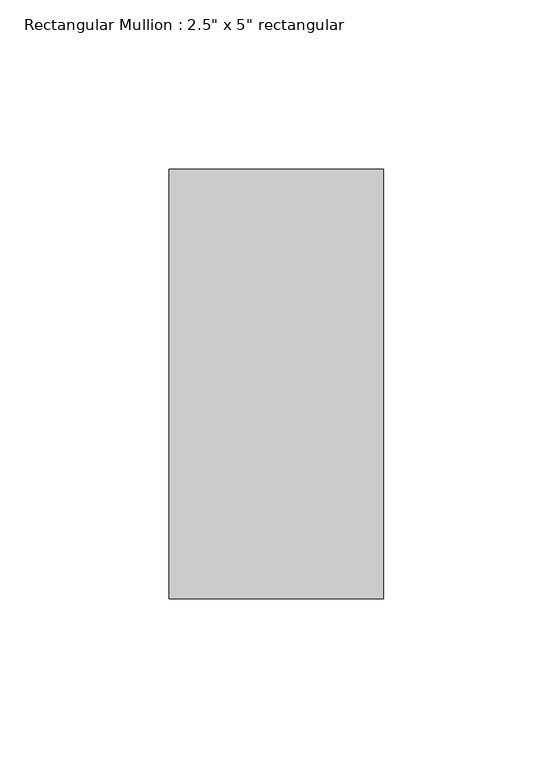
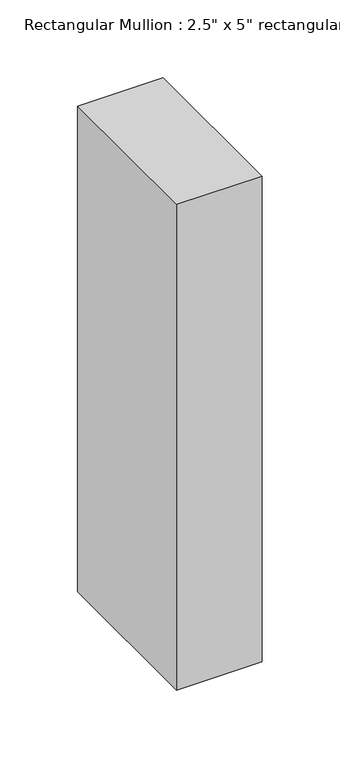
"""IFC4 building model written with IfcOpenShell, lengths in millimetres: member geometry."""

from ifc_helpers import new_model, si_unit, frame, origin, place, context, project, spatial, polyline, outline, extrude, source, transform, mapped, element, save


def member_03a502dc(model_context):
    return source(origin(), model_context, "Body", "SweptSolid", [
        extrude(outline(polyline([(31.75, 63.5), (31.75, -63.5), (-31.75, -63.5), (-31.75, 63.5), (31.75, 63.5)])), frame((0.0, 0.0, -381.0), z_axis=(0.0, 0.0, 1.0), x_axis=(1.0, 0.0, 0.0)), (0.0, 0.0, 1.0), 381.0),
    ])


if __name__ == "__main__":
    model = new_model("IFC4")
    model_context = context("Model", 3, world=origin())
    ifc_project = project(units=[si_unit("LENGTHUNIT", "METRE", prefix="MILLI")], contexts=[model_context])
    site = spatial("IfcSite", under=ifc_project)
    building = spatial("IfcBuilding", under=site)
    placement = place(None, origin())
    member_shape = member_03a502dc(model_context)
    element("IfcMember", 1, ObjectType="Rectangular Mullion : 2.5\" x 5\" rectangular", at=placement, inside=building, context=model_context, shape_type="MappedRepresentation", body=[
        mapped(member_shape, transform((0.0, 0.0, 0.0), x_axis=(1.0, 0.0, 0.0), y_axis=(0.0, 1.0, 0.0), z_axis=(0.0, 0.0, 1.0))),
    ])
    save(model, "model.ifc")

# Revit data of these elements
# Type "Rectangular Mullion : 2.5\" x 5\" rectangular"
#   built-in parameter 1007304 = 0.416667 (stored number, unit not read)
#   built-in parameter 1007301 = 0.104167 (stored number, unit not read)
#   built-in parameter 1007300 = 0.104167 (stored number, unit not read)
